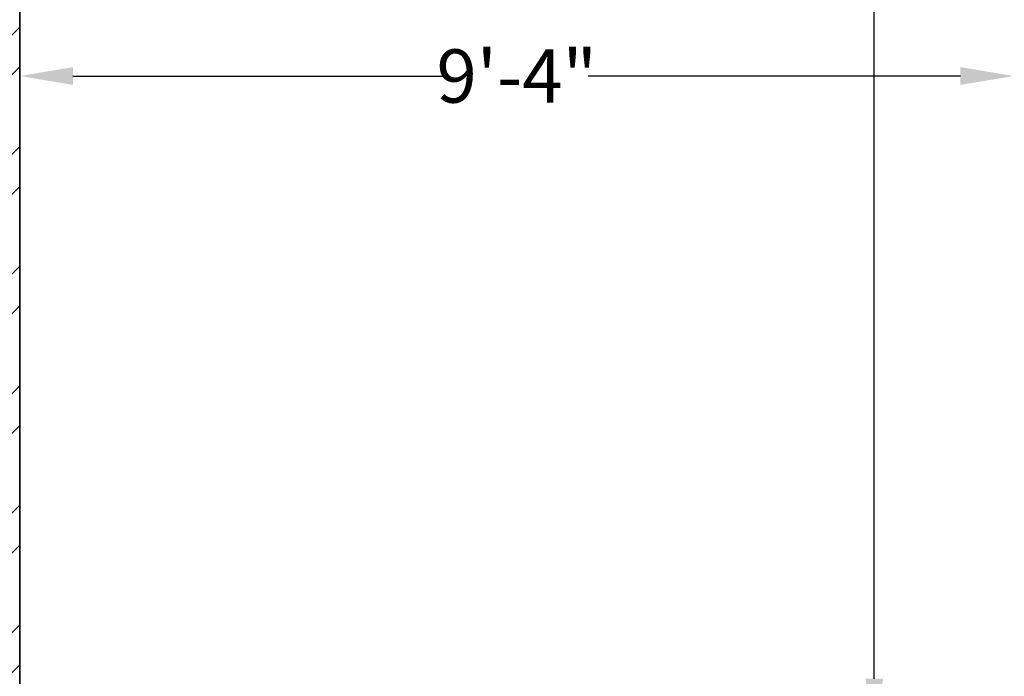
# Model space of a CAD drawing. Units: inches. Extents: x 3614 to 4242, y 2406 to 3033.
# Tile 3 of 10: x 3697 to 3808, y 2749 to 2823. Entities that reach past the tile are written whole.
import ezdxf

# ---------------------------------------------------------------- set-up
doc = ezdxf.new("R2010")
doc.units = ezdxf.units.IN
for name, color, linetype, lineweight in [('A-ANNO-DIMS', 2, 'Continuous', 18), ('A-WALL', 7, 'Continuous', 35), ('A-WALL-PATT', 252, 'Continuous', 13)]:
    doc.layers.add(name, color=color, linetype=linetype, lineweight=lineweight)
doc.styles.get("Standard").update_dxf_attribs({"font": 'arial.ttf'})
doc.dimstyles.get("Standard").update_dxf_attribs({"dimtxt": 6, "dimasz": 6, "dimexe": 0.18, "dimexo": 0.0625, "dimgap": 0.09, "dimtad": 0, "dimtih": 1, "dimtoh": 1, "dimdec": 4, "dimzin": 0, "dimdsep": 46, "dimlunit": 4, "dimtxsty": 'Standard', "dimcen": 0.09, "dimse1": 1, "dimse2": 1, "dimadec": 0, "dimazin": 0, "dimtfac": 1, "dimtdec": 4, "dimtofl": 0, "dimtmove": 0, "dimatfit": 3, "dimfxl": 1, "dimtolj": 1, "dimtzin": 0, "dimarcsym": 0})

# ---------------------------------------------------------------- blocks, each defined once
blk = doc.blocks.new('*D15')
at = {"layer": 'A-ANNO-DIMS', "color": 0, "lineweight": -2, "transparency": 16777216}
for p, q in [((3793.63, 2939.34), (3793.63, 2846.99)), ((3793.63, 2748.34), (3793.63, 2840.69))]:
    blk.add_line(p, q, dxfattribs=at)
at = {"layer": 'A-ANNO-DIMS', "color": 0, "transparency": 16777216}
for points in [[(3792.63, 2939.34), (3794.63, 2939.34), (3793.63, 2945.34)], [(3792.63, 2748.34), (3794.63, 2748.34), (3793.63, 2742.34)]]:
    blk.add_solid(points, dxfattribs=at)
at = {"layer": 'Defpoints', "color": 0, "transparency": 16777216}
for p in [(3799.84, 2945.34), (3793.63, 2742.34), (3799.84, 2742.34)]:
    blk.add_point(p, dxfattribs=at)
at = {"layer": 'A-ANNO-DIMS', "color": 0, "transparency": 16777216, "insert": (3793.63, 2843.84), "char_height": 6, "attachment_point": 5}
blk.add_mtext('\\A1;16\'-11"', dxfattribs=at)
blk = doc.blocks.new('*D16')
at = {"layer": 'A-ANNO-DIMS', "color": 0, "lineweight": -2, "transparency": 16777216}
for p, q in [((3703.34, 2816.24), (3745.27, 2816.24)), ((3803.34, 2816.24), (3761.4, 2816.24))]:
    blk.add_line(p, q, dxfattribs=at)
at = {"layer": 'A-ANNO-DIMS', "color": 0, "transparency": 16777216}
for points in [[(3703.34, 2817.24), (3703.34, 2815.24), (3697.34, 2816.24)], [(3803.34, 2817.24), (3803.34, 2815.24), (3809.34, 2816.24)]]:
    blk.add_solid(points, dxfattribs=at)
at = {"layer": 'Defpoints', "color": 0, "transparency": 16777216}
for p in [(3809.34, 2816.24), (3697.34, 2813.05), (3809.34, 2813.05)]:
    blk.add_point(p, dxfattribs=at)
at = {"layer": 'A-ANNO-DIMS', "color": 0, "transparency": 16777216, "insert": (3753.34, 2816.24), "char_height": 6, "attachment_point": 5}
blk.add_mtext('\\A1;9\'-4"', dxfattribs=at)

msp = doc.modelspace()

# ---------------------------------------------------------------- hatches: boundary and pattern name
at = {"layer": 'A-WALL-PATT'}
h = msp.add_hatch(dxfattribs=at)
h.set_pattern_fill('ANSI32', color=256)
h.paths.add_polyline_path([(4041.01458, 2954.34049), (3982.96188, 2954.34049), (3982.96188, 2945.34049), (3983.336, 2945.34049), (4041.01458, 2945.34049)])
h.paths.add_polyline_path([(3973.96188, 2954.34049), (3960.11861, 2954.34049), (3960.11861, 2945.34049), (3973.96188, 2945.34049)])
h.paths.add_polyline_path([(3936.11861, 2954.34049), (3901.17016, 2954.34049), (3901.17016, 2945.34049), (3913.336, 2945.34049), (3913.336, 2896.34049, -0.050382044), (3919.336, 2895.73437), (3919.336, 2945.34049), (3936.11861, 2945.34049)])
h.paths.add_polyline_path([(3983.336, 2945.34049), (3982.96188, 2945.34049), (3974.336, 2945.34049), (3974.336, 2873.34049), (3974.336, 2795.31105), (3983.336, 2795.31105), (3983.336, 2867.34049)])
h.paths.add_polyline_path([(3974.336, 2872.34049), (3919.336, 2872.34049), (3858.336, 2872.34049), (3858.336, 2866.34049), (3919.336, 2866.34049), (3974.336, 2866.34049)])
h.paths.add_polyline_path([(3877.17016, 2954.34049), (3852.34021, 2954.34049), (3852.34021, 2945.34049), (3852.336, 2896.34049), (3858.336, 2896.34049), (3858.336, 2945.34049), (3877.17016, 2945.34049)])
h.paths.add_polyline_path([(3871.94212, 2902.34049), (3858.336, 2902.34049), (3858.336, 2896.34049), (3871.336, 2896.34049, -0.050382044)], flags=0)
h.paths.add_polyline_path([(3913.336, 2902.34049), (3901.336, 2902.34049), (3901.336, 2896.34049), (3913.336, 2896.34049)], flags=17)
h.paths.add_polyline_path([(3858.336, 2872.34049), (3852.336, 2872.34049), (3852.336, 2866.34049), (3858.336, 2866.34049)])
h.paths.add_polyline_path([(3809.336, 2954.34049), (3764.4617, 2954.34049), (3764.4617, 2945.34049), (3809.336, 2945.34049)])
h.paths.add_polyline_path([(3716.4617, 2954.34049), (3697.336, 2954.34049), (3697.336, 2945.34049), (3716.4617, 2945.34049)])
h.paths.add_polyline_path([(3697.336, 2945.34049), (3688.336, 2945.34049), (3688.336, 2894.73438), (3697.336, 2894.73438)])
h = msp.add_hatch(dxfattribs=at)
h.set_pattern_fill('ANSI32', color=256)
h.paths.add_polyline_path([(4153.336, 2945.34049), (4144.336, 2945.34049), (4144.336, 2902.95478), (4153.336, 2902.95478)])
h.paths.add_polyline_path([(4144.36882, 2954.34049), (4089.01458, 2954.34049), (4089.01458, 2945.34049), (4144.36882, 2945.34049)])
h.paths.add_polyline_path([(3818.336, 2945.34049), (3809.336, 2945.34049), (3809.336, 2787.28572), (3818.336, 2787.28572)])
h.paths.add_polyline_path([(3697.336, 2846.73438), (3688.336, 2846.73438), (3688.336, 2742.34049), (3697.336, 2742.34049)])
h.paths.add_polyline_path([(3854.336, 2742.34049), (3853.36389, 2742.34049), (3818.336, 2742.34049), (3809.336, 2742.34049), (3697.336, 2742.34049), (3697.336, 2733.34049), (3809.336, 2733.34049), (3854.336, 2733.34049)])
h.paths.add_polyline_path([(3697.336, 2733.34049), (3688.336, 2733.34049), (3688.336, 2690.05693), (3697.336, 2690.05693)])
h.paths.add_polyline_path([(3697.336, 2642.05693), (3688.336, 2642.05693), (3688.336, 2583.37355), (3697.336, 2583.37355)])
h.paths.add_polyline_path([(3726.39802, 2583.34049), (3697.336, 2583.34049), (3697.336, 2574.34049), (3726.39802, 2574.34049)])
h.paths.add_polyline_path([(3842.336, 2583.34049), (3818.336, 2583.34049), (3809.336, 2583.34049), (3774.39802, 2583.34049), (3774.39802, 2574.34049), (3809.336, 2574.34049), (3842.336, 2574.34049)])
h.paths.add_polyline_path([(3890.336, 2583.34049), (3878.336, 2583.34049), (3878.336, 2574.34049), (3890.336, 2574.34049)])

# ---------------------------------------------------------------- linework, layer by layer
at = {"layer": 'A-WALL'}
msp.add_line((3697.336, 2945.34049), (3697.336, 2742.34049), dxfattribs=at)

# ---------------------------------------------------------------- dimensions: what is measured, and where the dimension line sits
at = {"layer": 'A-ANNO-DIMS'}
dim = msp.add_linear_dim(base=(3793.63235, 2742.34049), p1=(3799.84322, 2945.34049), p2=(3799.84322, 2742.34049), angle=90, dimstyle='Standard', override={"dimclrd": 0, "dimclre": 0, "dimclrt": 0}, dxfattribs=at)
dim.commit()
dim.dimension.update_dxf_attribs({"geometry": '*D15', "text_midpoint": (3793.63235, 2843.84049)})
dim = msp.add_linear_dim(base=(3809.336, 2816.23511), p1=(3697.336, 2813.04672), p2=(3809.336, 2813.04672), dimstyle='Standard', override={"dimclrd": 0, "dimclre": 0, "dimclrt": 0}, dxfattribs=at)
dim.commit()
dim.dimension.update_dxf_attribs({"geometry": '*D16', "text_midpoint": (3753.336, 2816.23511)})

doc.saveas('drawing.dxf')
